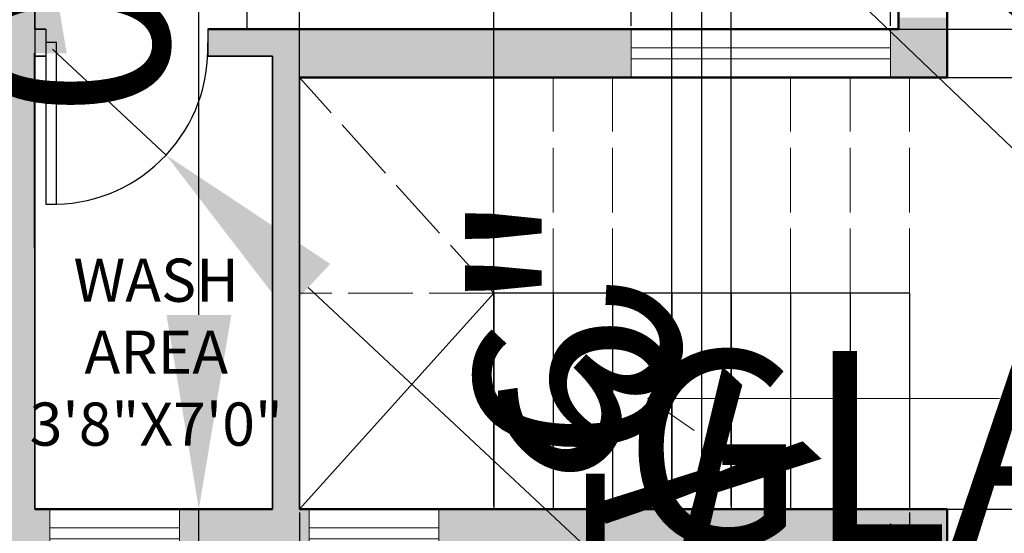
# Model space of a CAD drawing. Units: inches. Extents: x -299 to 1164, y -2 to 940.
# Tile 4 of 11: x 414 to 597, y 218 to 313. Entities that reach past the tile are written whole.
import ezdxf

# ---------------------------------------------------------------- set-up
doc = ezdxf.new("R2010")
doc.units = ezdxf.units.IN
doc.linetypes.add('ACAD_ISO02W100', pattern=[15, 12, -3])
for name, color, linetype, lineweight in [('A-ANNO-SYMB', 130, 'Continuous', 18), ('A-AREA-IDEN', 3, 'Continuous', 25), ('A-FLOR-CASE', 7, 'Continuous', 25), ('A-FLOR-STRS-OVHD', 6, 'ACAD_ISO02W100', 18), ('dimensions', 191, 'Continuous', 18), ('doors', 20, 'Continuous', 25), ('inner walls', 7, 'Continuous', 35), ('outer walls', 7, 'Continuous', 50), ('stairs', 6, 'Continuous', 25), ('windows', 130, 'Continuous', 18)]:
    doc.layers.add(name, color=color, linetype=linetype, lineweight=lineweight)
doc.layers.add('A-WALL-PATT', color=240, linetype='Continuous', lineweight=13, true_color=0xed1f24)
doc.styles.get("Standard").update_dxf_attribs({"font": 'arial.ttf'})
doc.dimstyles.new('ISO-25', dxfattribs={"dimtxt": 36, "dimasz": 36, "dimexe": 1.25, "dimexo": 0.625, "dimtad": 1, "dimlunit": 3, "dimtxsty": 'Standard', "dimcen": 2.5, "dimazin": 0, "dimtfac": 1, "dimtmove": 0, "dimatfit": 3, "dimfxl": 1, "dimarcsym": 0})

# ---------------------------------------------------------------- blocks, each defined once
blk = doc.blocks.new('glass')
at = {"layer": 'windows'}
for p, q in [((-12, 5.5), (-12, -3.5)), ((12, 5.5), (12, -3.5)), ((-12, 2), (12, 2)), ((-12, 0), (12, 0))]:
    blk.add_line(p, q, dxfattribs=at)
blk = doc.blocks.new('*D27')
at = {"layer": 'Defpoints', "color": 0, "transparency": 16777216}
for p in [(412.07, 375.49), (416.95, 375.49), (412.07, 342.99)]:
    blk.add_point(p, dxfattribs=at)
at = {"layer": 'dimensions', "color": 0, "lineweight": -2, "transparency": 16777216}
for p, q in [((416.95, 411.49), (416.95, 915.12)), ((412.7, 375.49), (418.2, 375.49)), ((416.95, 342.99), (416.95, 375.49)), ((412.7, 342.99), (418.2, 342.99)), ((416.95, 306.99), (416.95, 270.99))]:
    blk.add_line(p, q, dxfattribs=at)
at = {"layer": 'dimensions', "color": 0, "transparency": 16777216}
for points in [[(410.95, 411.49), (422.95, 411.49), (416.95, 375.49)], [(410.95, 306.99), (422.95, 306.99), (416.95, 342.99)]]:
    blk.add_solid(points, dxfattribs=at)
at = {"layer": 'dimensions', "color": 0, "transparency": 16777216, "insert": (397.69, 681.3), "char_height": 36, "attachment_point": 5, "rotation": 90}
blk.add_mtext('DOOR 2\'-8 1/2" TYP.', dxfattribs=at)
blk = doc.blocks.new('*D28')
at = {"layer": 'Defpoints', "color": 0, "transparency": 16777216}
for p in [(379.74, 342.99), (412.07, 342.99), (412.07, 338.11)]:
    blk.add_point(p, dxfattribs=at)
at = {"layer": 'dimensions', "color": 0, "lineweight": -2, "transparency": 16777216}
for p, q in [((379.74, 342.36), (379.74, 336.86)), ((412.07, 342.36), (412.07, 336.86)), ((343.74, 338.11), (307.74, 338.11)), ((379.74, 338.11), (412.07, 338.11)), ((448.07, 338.11), (789.26, 338.11))]:
    blk.add_line(p, q, dxfattribs=at)
at = {"layer": 'dimensions', "color": 0, "transparency": 16777216}
for points in [[(343.74, 344.11), (343.74, 332.11), (379.74, 338.11)], [(448.07, 344.11), (448.07, 332.11), (412.07, 338.11)]]:
    blk.add_solid(points, dxfattribs=at)
at = {"layer": 'dimensions', "color": 0, "transparency": 16777216, "insert": (636.66, 357.35), "char_height": 36, "attachment_point": 5}
blk.add_mtext('2\'-8 1/2" TYP.', dxfattribs=at)
blk = doc.blocks.new('*D29')
at = {"layer": 'Defpoints', "color": 0, "transparency": 16777216}
for p in [(304.07, 183.49), (376.07, 183.49), (376.07, 172.69)]:
    blk.add_point(p, dxfattribs=at)
at = {"layer": 'dimensions', "color": 0, "lineweight": -2, "transparency": 16777216}
for p, q in [((304.07, 182.86), (304.07, 171.44)), ((376.07, 182.86), (376.07, 171.44)), ((268.07, 172.69), (232.07, 172.69)), ((304.07, 172.69), (376.07, 172.69)), ((412.07, 172.69), (904.87, 172.69))]:
    blk.add_line(p, q, dxfattribs=at)
at = {"layer": 'dimensions', "color": 0, "transparency": 16777216}
for points in [[(268.07, 178.69), (268.07, 166.69), (304.07, 172.69)], [(412.07, 178.69), (412.07, 166.69), (376.07, 172.69)]]:
    blk.add_solid(points, dxfattribs=at)
at = {"layer": 'dimensions', "color": 0, "transparency": 16777216, "insert": (676.47, 191.94), "char_height": 36, "attachment_point": 5}
blk.add_mtext('WINDOW 6\'-0" TYP.', dxfattribs=at)
blk = doc.blocks.new('*D30')
at = {"layer": 'Defpoints', "color": 0, "transparency": 16777216}
for p in [(376.07, 192.49), (386.87, 192.49), (376.07, 183.49)]:
    blk.add_point(p, dxfattribs=at)
at = {"layer": 'dimensions', "color": 0, "lineweight": -2, "transparency": 16777216}
for p, q in [((386.87, 228.49), (386.87, 485.18)), ((376.7, 192.49), (388.12, 192.49)), ((386.87, 183.49), (386.87, 192.49)), ((376.7, 183.49), (388.12, 183.49)), ((386.87, 147.49), (386.87, 111.49))]:
    blk.add_line(p, q, dxfattribs=at)
at = {"layer": 'dimensions', "color": 0, "transparency": 16777216}
for points in [[(380.87, 228.49), (392.87, 228.49), (386.87, 192.49)], [(380.87, 147.49), (392.87, 147.49), (386.87, 183.49)]]:
    blk.add_solid(points, dxfattribs=at)
at = {"layer": 'dimensions', "color": 0, "transparency": 16777216, "insert": (367.87, 374.83), "char_height": 36, "attachment_point": 5, "rotation": 90}
blk.add_mtext('0\'-9" TYP.', dxfattribs=at)
blk = doc.blocks.new('*D33')
at = {"layer": 'Defpoints', "color": 0, "transparency": 16777216}
for p in [(419.84, 213.49), (443.84, 213.49), (443.84, 209.89)]:
    blk.add_point(p, dxfattribs=at)
at = {"layer": 'dimensions', "color": 0, "lineweight": -2, "transparency": 16777216}
for p, q in [((419.84, 212.86), (419.84, 208.64)), ((443.84, 212.86), (443.84, 208.64)), ((383.84, 209.89), (347.84, 209.89)), ((419.84, 209.89), (443.84, 209.89)), ((479.84, 209.89), (970.68, 209.89))]:
    blk.add_line(p, q, dxfattribs=at)
at = {"layer": 'dimensions', "color": 0, "transparency": 16777216}
for points in [[(383.84, 215.89), (383.84, 203.89), (419.84, 209.89)], [(479.84, 215.89), (479.84, 203.89), (443.84, 209.89)]]:
    blk.add_solid(points, dxfattribs=at)
at = {"layer": 'dimensions', "color": 0, "transparency": 16777216, "insert": (743.26, 229.13), "char_height": 36, "attachment_point": 5}
blk.add_mtext('GLAZING 2\'-0" TYP.', dxfattribs=at)
blk = doc.blocks.new('*D34')
at = {"layer": 'Defpoints', "color": 0, "transparency": 16777216}
for p in [(443.84, 222.49), (447.44, 222.49), (443.84, 213.49)]:
    blk.add_point(p, dxfattribs=at)
at = {"layer": 'dimensions', "color": 0, "lineweight": -2, "transparency": 16777216}
for p, q in [((447.44, 258.49), (447.44, 515.18)), ((444.47, 222.49), (448.69, 222.49)), ((447.44, 213.49), (447.44, 222.49)), ((444.47, 213.49), (448.69, 213.49)), ((447.44, 177.49), (447.44, 141.49))]:
    blk.add_line(p, q, dxfattribs=at)
at = {"layer": 'dimensions', "color": 0, "transparency": 16777216}
for points in [[(441.44, 258.49), (453.44, 258.49), (447.44, 222.49)], [(441.44, 177.49), (453.44, 177.49), (447.44, 213.49)]]:
    blk.add_solid(points, dxfattribs=at)
at = {"layer": 'dimensions', "color": 0, "transparency": 16777216, "insert": (428.44, 404.83), "char_height": 36, "attachment_point": 5, "rotation": 90}
blk.add_mtext('0\'-9" TYP.', dxfattribs=at)
blk = doc.blocks.new('*D37')
at = {"layer": 'Defpoints', "color": 0, "transparency": 16777216}
for p in [(588.07, 400.99), (624.7, 400.99), (624.7, 395.5)]:
    blk.add_point(p, dxfattribs=at)
at = {"layer": 'dimensions', "color": 0, "lineweight": -2, "transparency": 16777216}
for p, q in [((588.07, 400.36), (588.07, 394.25)), ((624.7, 400.36), (624.7, 394.25)), ((552.07, 395.5), (516.07, 395.5)), ((588.07, 395.5), (624.7, 395.5)), ((660.7, 395.5), (1164.33, 395.5))]:
    blk.add_line(p, q, dxfattribs=at)
at = {"layer": 'dimensions', "color": 0, "transparency": 16777216}
for points in [[(552.07, 401.5), (552.07, 389.5), (588.07, 395.5)], [(660.7, 401.5), (660.7, 389.5), (624.7, 395.5)]]:
    blk.add_solid(points, dxfattribs=at)
at = {"layer": 'dimensions', "color": 0, "transparency": 16777216, "insert": (930.51, 414.76), "char_height": 36, "attachment_point": 5}
blk.add_mtext('DOOR 3\'-0 1/2" TYP.', dxfattribs=at)
blk = doc.blocks.new('*D41')
at = {"layer": 'Defpoints', "color": 0, "transparency": 16777216}
for p in [(545.04, 388.33), (540.54, 358.33), (545.04, 358.33)]:
    blk.add_point(p, dxfattribs=at)
at = {"layer": 'dimensions', "color": 0, "lineweight": -2, "transparency": 16777216}
for p, q in [((540.54, 424.33), (540.54, 460.33)), ((544.41, 388.33), (539.29, 388.33)), ((540.54, 388.33), (540.54, 358.33)), ((544.41, 358.33), (539.29, 358.33)), ((540.54, 322.33), (540.54, -1.56))]:
    blk.add_line(p, q, dxfattribs=at)
at = {"layer": 'dimensions', "color": 0, "transparency": 16777216}
for points in [[(534.54, 424.33), (546.54, 424.33), (540.54, 388.33)], [(534.54, 322.33), (546.54, 322.33), (540.54, 358.33)]]:
    blk.add_solid(points, dxfattribs=at)
at = {"layer": 'dimensions', "color": 0, "transparency": 16777216, "insert": (521.3, 142.39), "char_height": 36, "attachment_point": 5, "rotation": 90}
blk.add_mtext('RANGE 2\'-6"', dxfattribs=at)
blk = doc.blocks.new('*D45')
at = {"layer": 'Defpoints', "color": 0, "transparency": 16777216}
for p in [(466.07, 222.49), (579.07, 222.49), (579.07, 127.99)]:
    blk.add_point(p, dxfattribs=at)
at = {"layer": 'dimensions', "color": 0, "lineweight": -2, "transparency": 16777216}
for p, q in [((466.07, 221.86), (466.07, 126.74)), ((579.07, 221.86), (579.07, 126.74)), ((502.07, 127.99), (543.07, 127.99))]:
    blk.add_line(p, q, dxfattribs=at)
at = {"layer": 'dimensions', "color": 0, "transparency": 16777216}
for points in [[(502.07, 133.99), (502.07, 121.99), (466.07, 127.99)], [(543.07, 133.99), (543.07, 121.99), (579.07, 127.99)]]:
    blk.add_solid(points, dxfattribs=at)
at = {"layer": 'dimensions', "color": 0, "transparency": 16777216, "insert": (522.57, 146.99), "char_height": 36, "attachment_point": 5}
blk.add_mtext('9\'-5"', dxfattribs=at)
blk = doc.blocks.new('*D46')
at = {"layer": 'Defpoints', "color": 0, "transparency": 16777216}
for p in [(579.07, 302.49), (770.93, 302.49), (579.07, 222.49)]:
    blk.add_point(p, dxfattribs=at)
at = {"layer": 'dimensions', "color": 0, "lineweight": -2, "transparency": 16777216}
for p, q in [((770.93, 302.49), (770.93, 435.63)), ((579.7, 302.49), (772.18, 302.49)), ((770.93, 258.49), (770.93, 266.49)), ((579.7, 222.49), (772.18, 222.49))]:
    blk.add_line(p, q, dxfattribs=at)
at = {"layer": 'dimensions', "color": 0, "transparency": 16777216}
for points in [[(764.93, 266.49), (776.93, 266.49), (770.93, 302.49)], [(764.93, 258.49), (776.93, 258.49), (770.93, 222.49)]]:
    blk.add_solid(points, dxfattribs=at)
at = {"layer": 'dimensions', "color": 0, "transparency": 16777216, "insert": (751.92, 387.06), "char_height": 36, "attachment_point": 5, "rotation": 90}
blk.add_mtext('6\'-8"', dxfattribs=at)
blk = doc.blocks.new('*D47')
at = {"layer": 'Defpoints', "color": 0, "transparency": 16777216}
for p in [(502.07, 668.99), (466.07, 222.49), (502.07, 222.49)]:
    blk.add_point(p, dxfattribs=at)
at = {"layer": 'dimensions', "color": 0, "lineweight": -2, "transparency": 16777216}
for p, q in [((466.07, 223.11), (466.07, 670.24)), ((502.07, 223.11), (502.07, 670.24)), ((430.07, 668.99), (394.07, 668.99)), ((466.07, 668.99), (502.07, 668.99)), ((538.07, 668.99), (670.99, 668.99))]:
    blk.add_line(p, q, dxfattribs=at)
at = {"layer": 'dimensions', "color": 0, "transparency": 16777216}
for points in [[(430.07, 674.99), (430.07, 662.99), (466.07, 668.99)], [(538.07, 674.99), (538.07, 662.99), (502.07, 668.99)]]:
    blk.add_solid(points, dxfattribs=at)
at = {"layer": 'dimensions', "color": 0, "transparency": 16777216, "insert": (622.53, 688.01), "char_height": 36, "attachment_point": 5}
blk.add_mtext('3\'-0"', dxfattribs=at)
blk = doc.blocks.new('*D48')
at = {"layer": 'Defpoints', "color": 0, "transparency": 16777216}
for p in [(546.07, 668.99), (535.07, 222.49), (546.07, 222.49)]:
    blk.add_point(p, dxfattribs=at)
at = {"layer": 'dimensions', "color": 0, "lineweight": -2, "transparency": 16777216}
for p, q in [((535.07, 223.11), (535.07, 670.24)), ((546.07, 223.11), (546.07, 670.24)), ((499.07, 668.99), (463.07, 668.99)), ((535.07, 668.99), (546.07, 668.99)), ((582.07, 668.99), (742.99, 668.99))]:
    blk.add_line(p, q, dxfattribs=at)
at = {"layer": 'dimensions', "color": 0, "transparency": 16777216}
for points in [[(499.07, 674.99), (499.07, 662.99), (535.07, 668.99)], [(582.07, 674.99), (582.07, 662.99), (546.07, 668.99)]]:
    blk.add_solid(points, dxfattribs=at)
at = {"layer": 'dimensions', "color": 0, "transparency": 16777216, "insert": (680.53, 687.99), "char_height": 36, "attachment_point": 5}
blk.add_mtext('0\'-11"', dxfattribs=at)
blk = doc.blocks.new('*D52')
at = {"layer": 'Defpoints', "color": 0, "transparency": 16777216}
for p in [(575.54, 668.99), (527.54, 311.49), (575.54, 311.49)]:
    blk.add_point(p, dxfattribs=at)
at = {"layer": 'dimensions', "color": 0, "lineweight": -2, "transparency": 16777216}
for p, q in [((527.54, 312.11), (527.54, 670.24)), ((575.54, 312.11), (575.54, 670.24)), ((491.54, 668.99), (455.54, 668.99)), ((527.54, 668.99), (575.54, 668.99)), ((611.54, 668.99), (745.94, 668.99))]:
    blk.add_line(p, q, dxfattribs=at)
at = {"layer": 'dimensions', "color": 0, "transparency": 16777216}
for points in [[(491.54, 674.99), (491.54, 662.99), (527.54, 668.99)], [(611.54, 674.99), (611.54, 662.99), (575.54, 668.99)]]:
    blk.add_solid(points, dxfattribs=at)
at = {"layer": 'dimensions', "color": 0, "transparency": 16777216, "insert": (696.74, 687.99), "char_height": 36, "attachment_point": 5}
blk.add_mtext('4\'-0"', dxfattribs=at)
blk = doc.blocks.new('*D58')
at = {"layer": 'Defpoints', "color": 0, "transparency": 16777216}
for p in [(456.35, 347.49), (770.93, 347.49), (456.35, 311.49)]:
    blk.add_point(p, dxfattribs=at)
at = {"layer": 'dimensions', "color": 0, "lineweight": -2, "transparency": 16777216}
for p, q in [((770.93, 383.49), (770.93, 516.41)), ((456.97, 347.49), (772.18, 347.49)), ((770.93, 311.49), (770.93, 347.49)), ((456.97, 311.49), (772.18, 311.49)), ((770.93, 275.49), (770.93, 239.49))]:
    blk.add_line(p, q, dxfattribs=at)
at = {"layer": 'dimensions', "color": 0, "transparency": 16777216}
for points in [[(764.93, 383.49), (776.93, 383.49), (770.93, 347.49)], [(764.93, 275.49), (776.93, 275.49), (770.93, 311.49)]]:
    blk.add_solid(points, dxfattribs=at)
at = {"layer": 'dimensions', "color": 0, "transparency": 16777216, "insert": (751.91, 467.95), "char_height": 36, "attachment_point": 5, "rotation": 90}
blk.add_mtext('3\'-0"', dxfattribs=at)
blk = doc.blocks.new('*D59')
at = {"layer": 'Defpoints', "color": 0, "transparency": 16777216}
for p in [(697.05, 194.59), (730.81, 162.24)]:
    blk.add_point(p, dxfattribs=at)
at = {"layer": 'dimensions', "color": 0, "lineweight": -2, "transparency": 16777216}
for p, q in [((530.01, 354.68), (671.06, 219.5)), ((730.81, 162.24), (697.05, 194.59))]:
    blk.add_line(p, q, dxfattribs=at)
at = {"layer": 'dimensions', "color": 0, "transparency": 16777216}
blk.add_solid([(675.21, 223.83), (666.91, 215.17), (697.05, 194.59)], dxfattribs=at)
at = {"layer": 'dimensions', "color": 0, "transparency": 16777216, "insert": (600.7, 313.27), "char_height": 36, "attachment_point": 5, "rotation": 316.2186}
blk.add_mtext('R3\'-11"', dxfattribs=at)
blk = doc.blocks.new('*D62')
at = {"layer": 'Defpoints', "color": 0, "transparency": 16777216}
for p in [(420.34, 307.74), (441.36, 288.12)]:
    blk.add_point(p, dxfattribs=at)
at = {"layer": 'dimensions', "color": 0, "lineweight": -2, "transparency": 16777216}
for p, q in [((420.34, 307.74), (441.36, 288.12)), ((646.59, 96.57), (467.68, 263.55))]:
    blk.add_line(p, q, dxfattribs=at)
at = {"layer": 'dimensions', "color": 0, "transparency": 16777216}
blk.add_solid([(471.78, 267.94), (463.59, 259.17), (441.36, 288.12)], dxfattribs=at)
at = {"layer": 'dimensions', "color": 0, "transparency": 16777216, "insert": (583.27, 181.68), "char_height": 36, "attachment_point": 5, "rotation": 316.9755}
blk.add_mtext('3X R2\'-5"', dxfattribs=at)

msp = doc.modelspace()

# ---------------------------------------------------------------- hatches: boundary and pattern name
at = {"layer": 'A-WALL-PATT'}
h = msp.add_hatch(color=256, dxfattribs=at)
h.dxf.hatch_style = 1
h.paths.add_polyline_path([(312.071, 460.489), (307.071, 460.489), (307.071, 432.489), (307.071, 427.489), (372.071, 427.489), (372.071, 375.489), (372.071, 370.489), (380.071, 370.489, -0.0217424), (380.071, 372.989), (380.071, 375.489), (377.071, 375.489), (377.071, 427.489), (417.071, 427.489), (417.071, 489.489), (412.071, 489.489), (412.071, 484.489), (412.071, 432.489), (312.071, 432.489)], flags=17)
h.paths.add_polyline_path([(340.071, 372.989, -0.0217424), (340.071, 375.489), (268.071, 375.489), (268.071, 427.489), (268.071, 432.489), (268.071, 484.489), (268.071, 489.489), (268.071, 629.489), (412.071, 629.489), (412.071, 527.563, -0.0185322), (414.571, 527.489), (417.071, 527.489), (417.071, 629.489), (581.071, 629.489), (581.071, 553.489), (586.071, 553.489), (586.071, 629.489), (730.071, 629.489), (730.071, 405.489), (713.071, 405.489), (713.071, 396.489), (739.071, 396.489), (739.071, 638.489), (259.071, 638.489), (259.071, 183.489), (304.071, 183.489), (304.071, 192.489), (268.071, 192.489), (268.071, 370.489), (340.071, 370.489)])
h.paths.add_polyline_path([(417.071, 188.489), (417.071, 213.489), (461.071, 213.489), (461.071, 188.489)], flags=16)
h.paths.add_polyline_path([(586.071, 313.578), (577.071, 313.578), (577.071, 311.489), (575.54, 311.489), (575.54, 302.489), (586.071, 302.489)], flags=16)
h.paths.add_polyline_path([(586.071, 405.489), (586.071, 481.489), (581.071, 481.489), (581.071, 432.489), (499.071, 432.489), (499.071, 427.489), (577.071, 427.489), (577.071, 385.578), (586.071, 385.578), (586.071, 396.489)], flags=17)
h.paths.add_polyline_path([(641.071, 405.489), (624.071, 405.489, -0.0333689), (624.071, 400.989), (624.071, 396.489), (641.071, 396.489)], flags=17)
h.paths.add_polyline_path([(491.866, 222.489), (491.866, 213.489), (586.071, 213.489), (586.071, 222.489)])
edge = h.paths.add_edge_path()
edge.add_line((467.866, 213.489), (467.866, 222.489))
edge.add_line((467.866, 222.489), (466.071, 222.489))
edge.add_line((466.071, 222.489), (466.071, 302.489))
edge.add_line((466.071, 302.489), (527.54, 302.489))
edge.add_line((527.54, 302.489), (527.54, 311.489))
edge.add_line((527.54, 311.489), (449.071, 311.489))
edge.add_line((449.071, 311.489), (449.071, 308.989))
edge.add_arc((420.339, 307.739), 28.759, -2.4911, 2.4911, ccw=False)
edge.add_line((449.071, 306.489), (461.071, 306.489))
edge.add_line((461.071, 306.489), (461.071, 222.489))
edge.add_line((461.071, 222.489), (443.844, 222.489))
edge.add_line((443.844, 222.489), (443.844, 213.489))
edge.add_line((443.844, 213.489), (419.844, 213.489))
edge.add_line((419.844, 213.489), (419.844, 222.489))
edge.add_line((419.844, 222.489), (417.071, 222.489))
edge.add_line((417.071, 222.489), (417.071, 306.489))
edge.add_line((417.071, 306.489), (417.071, 311.489))
edge.add_line((417.071, 311.489), (417.071, 375.489))
edge.add_line((417.071, 375.489), (412.071, 375.489))
edge.add_line((412.071, 375.489), (412.071, 370.489))
edge.add_line((412.071, 370.489), (412.071, 192.489))
edge.add_line((412.071, 192.489), (376.071, 192.489))
edge.add_line((376.071, 192.489), (376.071, 183.489))
edge.add_line((376.071, 183.489), (412.071, 183.489))
edge.add_line((412.071, 183.489), (466.071, 183.489))
edge.add_line((466.071, 183.489), (466.071, 213.489))
edge.add_line((466.071, 213.489), (467.866, 213.489))

# ---------------------------------------------------------------- linework, layer by layer
at = {"layer": 'A-ANNO-SYMB'}
for p, q in [((539.197, 248.414), (530.621, 242.98)), ((595.785, 242.98), (530.621, 242.98)), ((530.621, 242.98), (536.549, 242.98)), ((530.621, 242.98), (539.197, 237.083))]:
    msp.add_line(p, q, dxfattribs=at)
at = {"layer": 'A-FLOR-CASE'}
msp.add_line((456.348, 347.489), (456.348, 311.489), dxfattribs=at)
at = {"layer": 'A-FLOR-STRS-OVHD'}
for p, q in [((502.071, 262.489), (466.071, 302.489)), ((502.071, 262.489), (502.071, 302.489)), ((513.071, 262.489), (513.071, 302.489)), ((524.071, 262.489), (524.071, 302.489)), ((535.071, 262.489), (535.071, 302.489)), ((546.071, 262.489), (546.071, 302.489)), ((557.071, 262.489), (557.071, 302.489)), ((568.071, 262.489), (568.071, 302.489)), ((579.071, 262.489), (579.071, 302.489)), ((502.071, 262.489), (466.071, 262.489))]:
    msp.add_line(p, q, dxfattribs=at)
at = {"layer": 'doors'}
for p, q in [((417.071, 311.489), (417.071, 306.489)), ((419.071, 311.489), (419.071, 306.489)), ((449.071, 311.489), (449.071, 306.489))]:
    msp.add_line(p, q, dxfattribs=at)
msp.add_lwpolyline([(419.071, 278.989), (421.071, 278.989), (421.071, 308.989), (419.071, 308.989)], close=True, dxfattribs=at)
msp.add_arc((420.339, 307.739), 28.759, 271.45877, 2.4911, dxfattribs=at)
at = {"layer": 'inner walls'}
for p, q in [((417.071, 375.489), (417.071, 311.489)), ((419.071, 311.489), (417.071, 311.489)), ((417.071, 306.489), (417.071, 222.489)), ((419.071, 306.489), (417.071, 306.489)), ((461.071, 306.489), (449.071, 306.489)), ((461.071, 306.489), (461.071, 222.489)), ((466.071, 302.489), (466.071, 222.489))]:
    msp.add_line(p, q, dxfattribs=at)
at = {"layer": 'outer walls'}
for p, q in [((577.071, 427.489), (577.071, 311.489)), ((586.071, 396.489), (586.071, 302.489)), ((577.071, 311.489), (449.071, 311.489)), ((586.071, 302.489), (466.071, 302.489)), ((461.071, 222.489), (417.071, 222.489)), ((586.071, 222.489), (466.071, 222.489)), ((586.071, 222.489), (586.071, 213.489))]:
    msp.add_line(p, q, dxfattribs=at)
at = {"layer": 'stairs'}
for p, q in [((502.071, 262.489), (466.071, 222.489)), ((579.071, 262.489), (502.071, 262.489)), ((502.071, 262.489), (502.071, 222.489)), ((513.071, 262.489), (513.071, 222.489)), ((524.071, 262.489), (524.071, 222.489)), ((535.071, 262.489), (535.071, 222.489)), ((546.071, 262.489), (546.071, 222.489)), ((557.071, 262.489), (557.071, 222.489)), ((568.071, 262.489), (568.071, 222.489)), ((579.071, 262.489), (579.071, 222.489))]:
    msp.add_line(p, q, dxfattribs=at)
at = {"layer": 'windows'}
for p, q in [((527.54, 307.989), (575.54, 307.989)), ((527.54, 305.989), (575.54, 305.989))]:
    msp.add_line(p, q, dxfattribs=at)
msp.add_lwpolyline([(527.54, 302.489), (575.54, 302.489), (575.54, 311.489), (527.54, 311.489)], close=True, dxfattribs=at)

# ---------------------------------------------------------------- block references
for p in [(431.844, 216.989), (479.866, 216.989)]:
    msp.add_blockref('glass', p, dxfattribs=at)

# ---------------------------------------------------------------- texts
at = {"layer": 'A-AREA-IDEN', "insert": (404.627, 268.912), "char_height": 8, "attachment_point": 1}
msp.add_mtext_dynamic_manual_height_columns('\\pxqc,t15;WASH\\PAREA\\P3\'8"X7\'0"', width=69.83809, gutter_width=12.5, heights=[0], dxfattribs=at)

# ---------------------------------------------------------------- dimensions: what is measured, and where the dimension line sits
at = {"layer": 'dimensions'}
for base, p1, p2, angle, text, picture, middle in [((416.946, 375.489), (412.071, 342.989), (412.071, 375.489), 90, 'DOOR <> TYP.', '*D27', (397.695, 681.304)), ((447.444, 222.489), (443.844, 213.489), (443.844, 222.489), 90, '<> TYP.', '*D34', (428.438, 404.833)), ((386.871, 192.489), (376.071, 183.489), (376.071, 192.489), 90, '<> TYP.', '*D30', (367.865, 374.833)), ((540.536, 358.335), (545.036, 388.335), (545.036, 358.335), 270, 'RANGE <>', '*D41', (521.297, 142.385))]:
    dim = msp.add_linear_dim(base=base, p1=p1, p2=p2, angle=angle, text=text, dimstyle='ISO-25', override={"dimdec": 1, "dimlfac": 1, "dimrnd": 0, "dimzin": 1, "dimdsep": 46, "dimlunit": 4, "dimfrac": 2}, dxfattribs=at)
    dim.commit()
    dim.dimension.update_dxf_attribs({"geometry": picture, "text_midpoint": middle})
for base, p1, p2, picture, middle in [((502.071, 668.989), (466.071, 222.489), (502.071, 222.489), '*D47', (622.532, 688.007)), ((575.54, 668.989), (527.54, 311.489), (575.54, 311.489), '*D52', (696.738, 687.995)), ((546.071, 668.989), (535.071, 222.489), (546.071, 222.489), '*D48', (680.53, 687.995)), ((579.071, 127.989), (466.071, 222.489), (579.071, 222.489), '*D45', (522.571, 146.995))]:
    dim = msp.add_linear_dim(base=base, p1=p1, p2=p2, dimstyle='ISO-25', override={"dimdec": 1, "dimlfac": 1, "dimrnd": 0, "dimzin": 1, "dimdsep": 46, "dimlunit": 4, "dimfrac": 2}, dxfattribs=at)
    dim.commit()
    dim.dimension.update_dxf_attribs({"geometry": picture, "text_midpoint": middle})
for base, p1, p2, text, picture, middle in [((624.698, 395.495), (588.071, 400.989), (624.698, 400.989), 'DOOR <> TYP.', '*D37', (930.512, 414.759)), ((412.071, 338.114), (379.736, 342.989), (412.071, 342.989), '<> TYP.', '*D28', (636.665, 357.353)), ((443.844, 209.889), (419.844, 213.489), (443.844, 213.489), 'GLAZING <> TYP.', '*D33', (743.261, 229.128)), ((376.071, 172.689), (304.071, 183.489), (376.071, 183.489), 'WINDOW <> TYP.', '*D29', (676.471, 191.94))]:
    dim = msp.add_linear_dim(base=base, p1=p1, p2=p2, text=text, dimstyle='ISO-25', override={"dimdec": 1, "dimlfac": 1, "dimrnd": 0, "dimzin": 1, "dimdsep": 46, "dimlunit": 4, "dimfrac": 2}, dxfattribs=at)
    dim.commit()
    dim.dimension.update_dxf_attribs({"geometry": picture, "text_midpoint": middle})
for base, p1, p2, picture, middle in [((770.929, 347.489), (456.348, 311.489), (456.348, 347.489), '*D58', (751.911, 467.95)), ((770.929, 302.489), (579.071, 222.489), (579.071, 302.489), '*D46', (751.923, 387.061))]:
    dim = msp.add_linear_dim(base=base, p1=p1, p2=p2, angle=90, dimstyle='ISO-25', override={"dimdec": 1, "dimlfac": 1, "dimrnd": 0, "dimzin": 1, "dimdsep": 46, "dimlunit": 4, "dimfrac": 2}, dxfattribs=at)
    dim.commit()
    dim.dimension.update_dxf_attribs({"geometry": picture, "text_midpoint": middle})
dim = msp.add_radius_dim(center=(730.81, 162.239), mpoint=(697.053, 194.59), dimstyle='ISO-25', override={"dimdec": 1, "dimlfac": 1, "dimrnd": 0, "dimzin": 1, "dimdsep": 46, "dimlunit": 4, "dimfrac": 2}, dxfattribs=at)
dim.commit()
dim.dimension.update_dxf_attribs({"geometry": '*D59', "text_midpoint": (600.698, 313.273)})
dim = msp.add_radius_dim(center=(420.339, 307.739), mpoint=(441.364, 288.116), text='3X <>', dimstyle='ISO-25', override={"dimdec": 1, "dimlfac": 1, "dimrnd": 0, "dimzin": 1, "dimdsep": 46, "dimlunit": 4, "dimfrac": 2}, dxfattribs=at)
dim.commit()
dim.dimension.update_dxf_attribs({"geometry": '*D62', "text_midpoint": (583.273, 181.684)})

doc.saveas('drawing.dxf')
